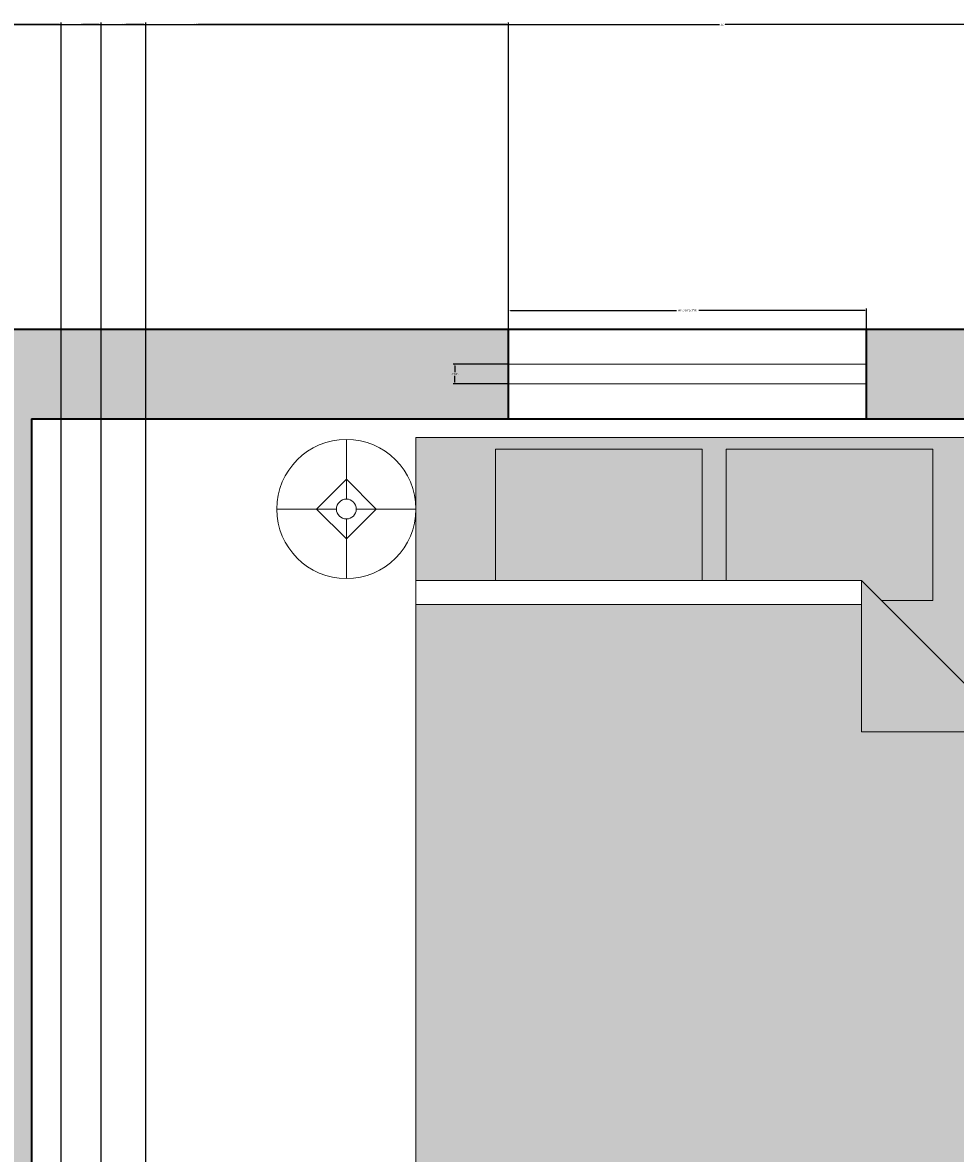
# Model space of a CAD drawing. Units: inches. Extents: x 1567 to 1964, y 1813 to 2447.
# Tile 27 of 28: x 1792 to 1885, y 2333 to 2447. Entities that reach past the tile are written whole.
import ezdxf

# ---------------------------------------------------------------- set-up
doc = ezdxf.new("R2010")
doc.units = ezdxf.units.IN
for name, color, linetype, lineweight in [('A-ANNO-DIMS', 2, 'Continuous', 18), ('A-FURN', 8, 'Continuous', 18), ('A-GLAZ', 4, 'Continuous', 18), ('A-WALL', 7, 'Continuous', 35)]:
    doc.layers.add(name, color=color, linetype=linetype, lineweight=lineweight)
doc.layers.add('A-FURN-PATT', color=252, linetype='Continuous', lineweight=13, true_color=0x939598)
doc.layers.add('A-WALL-PATT', color=251, linetype='Continuous', lineweight=13, true_color=0x636466)
doc.styles.get("Standard").update_dxf_attribs({"font": 'arial.ttf'})
doc.dimstyles.get("Standard").update_dxf_attribs({"dimtxt": 0.18, "dimasz": 0.18, "dimexe": 0.18, "dimexo": 0.0625, "dimgap": 0.09, "dimtad": 0, "dimtih": 1, "dimtoh": 1, "dimdec": 4, "dimzin": 0, "dimdsep": 46, "dimtxsty": 'Standard', "dimcen": 0.09, "dimadec": 0, "dimazin": 0, "dimtfac": 1, "dimtdec": 4, "dimtofl": 0, "dimtmove": 0, "dimatfit": 3, "dimfxl": 1, "dimtolj": 1, "dimtzin": 0, "dimarcsym": 0})

# ---------------------------------------------------------------- blocks, each defined once
blk = doc.blocks.new('Lamp - Table')
for p, q in [((0, 7), (0, 1)), ((0, 3), (-3, 0)), ((3, 0), (0, 3)), ((-1, 0), (-7, 0)), ((-3, 0), (0, -3)), ((0, -3), (3, 0)), ((1, 0), (7, 0)), ((0, -1), (0, -7))]:
    blk.add_line(p, q)
for radius in [7, 1]:
    blk.add_circle((0, 0), radius)
blk = doc.blocks.new('Bed - Queen')
for p, q in [((0, -80.00003), (0, 0)), ((0, 0), (59.99999, 0)), ((59.99999, 0), (59.99999, -80.00003)), ((7.99999, -1.2), (28.79998, -1.2)), ((7.99999, -14.4), (7.99999, -1.2)), ((28.79998, -1.2), (28.79998, -14.4)), ((31.19999, -1.2), (51.99999, -1.2)), ((31.19999, -14.4), (31.19999, -1.2)), ((51.99999, -1.2), (51.99999, -16.4)), ((0, -14.4), (44.8, -14.4)), ((59.99999, -29.6), (44.8, -14.4)), ((44.8, -14.4), (44.8, -29.6)), ((44.8, -16.8), (0, -16.8)), ((51.99999, -16.4), (46.79936, -16.4)), ((44.8, -29.6), (59.99999, -29.6)), ((59.99999, -80.00003), (0, -80.00003))]:
    blk.add_line(p, q)
blk = doc.blocks.new('WINDOW-36IN')
for p, q in [((0, 2), (36, 2)), ((0, 0), (36, 0))]:
    blk.add_line(p, q)
blk = doc.blocks.new('*D33')
at = {"layer": 'A-ANNO-DIMS', "color": 0, "lineweight": -2, "transparency": 16777216}
for p, q in [((1840.43, 2412.85), (1840.43, 2418.37)), ((1840.61, 2418.19), (1857.31, 2418.19)), ((1876.25, 2418.19), (1859.55, 2418.19)), ((1876.43, 2412.85), (1876.43, 2418.37))]:
    blk.add_line(p, q, dxfattribs=at)
at = {"layer": 'A-ANNO-DIMS', "color": 0, "transparency": 16777216}
for points in [[(1840.61, 2418.22), (1840.61, 2418.16), (1840.43, 2418.19)], [(1876.25, 2418.22), (1876.25, 2418.16), (1876.43, 2418.19)]]:
    blk.add_solid(points, dxfattribs=at)
at = {"layer": 'Defpoints', "color": 0, "transparency": 16777216}
for p in [(1840.43, 2418.19), (1840.43, 2412.79), (1876.43, 2412.79)]:
    blk.add_point(p, dxfattribs=at)
at = {"layer": 'A-ANNO-DIMS', "color": 0, "transparency": 16777216, "insert": (1858.43, 2418.19), "char_height": 0.18, "attachment_point": 5}
blk.add_mtext('\\A1;WINDOW 36 TYP.', dxfattribs=at)
blk = doc.blocks.new('*D34')
at = {"layer": 'A-ANNO-DIMS', "color": 0, "lineweight": -2, "transparency": 16777216}
for p, q in [((1840.37, 2412.79), (1834.85, 2412.79)), ((1835.03, 2412.61), (1835.03, 2411.97)), ((1835.03, 2410.97), (1835.03, 2411.61)), ((1840.37, 2410.79), (1834.85, 2410.79))]:
    blk.add_line(p, q, dxfattribs=at)
at = {"layer": 'A-ANNO-DIMS', "color": 0, "transparency": 16777216}
for points in [[(1835, 2412.61), (1835.06, 2412.61), (1835.03, 2412.79)], [(1835, 2410.97), (1835.06, 2410.97), (1835.03, 2410.79)]]:
    blk.add_solid(points, dxfattribs=at)
at = {"layer": 'Defpoints', "color": 0, "transparency": 16777216}
for p in [(1840.43, 2412.79), (1835.03, 2410.79), (1840.43, 2410.79)]:
    blk.add_point(p, dxfattribs=at)
at = {"layer": 'A-ANNO-DIMS', "color": 0, "transparency": 16777216, "insert": (1835.03, 2411.79), "char_height": 0.18, "attachment_point": 5}
blk.add_mtext('\\A1;2 TYP.', dxfattribs=at)
blk = doc.blocks.new('*D45')
at = {"layer": 'A-ANNO-DIMS', "color": 0, "lineweight": -2, "transparency": 16777216}
for p, q in [((1777.43, 2416.35), (1777.43, 2447.12)), ((1777.61, 2446.94), (1808.71, 2446.94)), ((1840.25, 2446.94), (1809.15, 2446.94)), ((1840.43, 2416.35), (1840.43, 2447.12))]:
    blk.add_line(p, q, dxfattribs=at)
at = {"layer": 'A-ANNO-DIMS', "color": 0, "transparency": 16777216}
for points in [[(1777.61, 2446.97), (1777.61, 2446.91), (1777.43, 2446.94)], [(1840.25, 2446.97), (1840.25, 2446.91), (1840.43, 2446.94)]]:
    blk.add_solid(points, dxfattribs=at)
at = {"layer": 'Defpoints', "color": 0, "transparency": 16777216}
for p in [(1840.43, 2446.94), (1777.43, 2416.29), (1840.43, 2416.29)]:
    blk.add_point(p, dxfattribs=at)
at = {"layer": 'A-ANNO-DIMS', "color": 0, "transparency": 16777216, "insert": (1808.93, 2446.94), "char_height": 0.18, "attachment_point": 5}
blk.add_mtext('\\A1;63', dxfattribs=at)
blk = doc.blocks.new('*D54')
at = {"layer": 'A-ANNO-DIMS', "color": 0, "lineweight": -2, "transparency": 16777216}
for p, q in [((1711.43, 1964.35), (1711.43, 2447.12)), ((1711.61, 2446.94), (1753.21, 2446.94)), ((1795.25, 2446.94), (1753.65, 2446.94)), ((1795.43, 1964.35), (1795.43, 2447.12))]:
    blk.add_line(p, q, dxfattribs=at)
at = {"layer": 'A-ANNO-DIMS', "color": 0, "transparency": 16777216}
for points in [[(1711.61, 2446.97), (1711.61, 2446.91), (1711.43, 2446.94)], [(1795.25, 2446.97), (1795.25, 2446.91), (1795.43, 2446.94)]]:
    blk.add_solid(points, dxfattribs=at)
at = {"layer": 'Defpoints', "color": 0, "transparency": 16777216}
for p in [(1795.43, 2446.94), (1711.43, 1964.29), (1795.43, 1964.29)]:
    blk.add_point(p, dxfattribs=at)
at = {"layer": 'A-ANNO-DIMS', "color": 0, "transparency": 16777216, "insert": (1753.43, 2446.94), "char_height": 0.18, "attachment_point": 5}
blk.add_mtext('\\A1;84', dxfattribs=at)
blk = doc.blocks.new('*D55')
at = {"layer": 'A-ANNO-DIMS', "color": 0, "lineweight": -2, "transparency": 16777216}
for p, q in [((1795.43, 1964.35), (1795.43, 2447.12)), ((1795.61, 2446.94), (1797.28, 2446.94)), ((1799.25, 2446.94), (1797.58, 2446.94)), ((1799.43, 1967.35), (1799.43, 2447.12))]:
    blk.add_line(p, q, dxfattribs=at)
at = {"layer": 'A-ANNO-DIMS', "color": 0, "transparency": 16777216}
for points in [[(1795.61, 2446.97), (1795.61, 2446.91), (1795.43, 2446.94)], [(1799.25, 2446.97), (1799.25, 2446.91), (1799.43, 2446.94)]]:
    blk.add_solid(points, dxfattribs=at)
at = {"layer": 'Defpoints', "color": 0, "transparency": 16777216}
for p in [(1799.43, 2446.94), (1799.43, 1967.29), (1795.43, 1964.29)]:
    blk.add_point(p, dxfattribs=at)
at = {"layer": 'A-ANNO-DIMS', "color": 0, "transparency": 16777216, "insert": (1797.43, 2446.94), "char_height": 0.18, "attachment_point": 5}
blk.add_mtext('\\A1;4', dxfattribs=at)
blk = doc.blocks.new('*D70')
at = {"layer": 'A-ANNO-DIMS', "color": 0, "lineweight": -2, "transparency": 16777216}
for p, q in [((1799.43, 1967.35), (1799.43, 2447.12)), ((1799.61, 2446.94), (1801.42, 2446.94)), ((1803.75, 2446.94), (1801.94, 2446.94)), ((1803.93, 1967.35), (1803.93, 2447.12))]:
    blk.add_line(p, q, dxfattribs=at)
at = {"layer": 'A-ANNO-DIMS', "color": 0, "transparency": 16777216}
for points in [[(1799.61, 2446.97), (1799.61, 2446.91), (1799.43, 2446.94)], [(1803.75, 2446.97), (1803.75, 2446.91), (1803.93, 2446.94)]]:
    blk.add_solid(points, dxfattribs=at)
at = {"layer": 'Defpoints', "color": 0, "transparency": 16777216}
for p in [(1803.93, 2446.94), (1799.43, 1967.29), (1803.93, 1967.29)]:
    blk.add_point(p, dxfattribs=at)
at = {"layer": 'A-ANNO-DIMS', "color": 0, "transparency": 16777216, "insert": (1801.68, 2446.94), "char_height": 0.18, "attachment_point": 5}
blk.add_mtext('\\A1;4.5', dxfattribs=at)
blk = doc.blocks.new('*D71')
at = {"layer": 'A-ANNO-DIMS', "color": 0, "lineweight": -2, "transparency": 16777216}
for p, q in [((1799.43, 1910.75), (1799.43, 2447.12)), ((1799.61, 2446.94), (1861.65, 2446.94)), ((1924.25, 2446.94), (1862.21, 2446.94)), ((1924.43, 1910.75), (1924.43, 2447.12))]:
    blk.add_line(p, q, dxfattribs=at)
at = {"layer": 'A-ANNO-DIMS', "color": 0, "transparency": 16777216}
for points in [[(1799.61, 2446.97), (1799.61, 2446.91), (1799.43, 2446.94)], [(1924.25, 2446.97), (1924.25, 2446.91), (1924.43, 2446.94)]]:
    blk.add_solid(points, dxfattribs=at)
at = {"layer": 'Defpoints', "color": 0, "transparency": 16777216}
for p in [(1924.43, 2446.94), (1799.43, 1910.69), (1924.43, 1910.69)]:
    blk.add_point(p, dxfattribs=at)
at = {"layer": 'A-ANNO-DIMS', "color": 0, "transparency": 16777216, "insert": (1861.93, 2446.94), "char_height": 0.18, "attachment_point": 5}
blk.add_mtext('\\A1;125', dxfattribs=at)

msp = doc.modelspace()

# ---------------------------------------------------------------- hatches: boundary and pattern name
at = {"layer": 'A-FURN-PATT'}
h = msp.add_hatch(color=256, dxfattribs=at)
h.dxf.hatch_style = 1
h.paths.add_polyline_path([(1621.2532, 2242.0229), (1643.7811, 2241.7239), (1643.8607, 2247.7234), (1617.863, 2248.0685, 0.19047621), (1616.7481, 2164.0759), (1642.7458, 2163.7308), (1642.8254, 2169.7302), (1620.2975, 2170.0293, -0.15194781)])
h.paths.add_polyline_path([(1673.5306, 2249.6607), (1653.8509, 2249.6607), (1653.8509, 2248.5031, 0.11764706), (1673.5306, 2248.5031)])
h.paths.add_polyline_path([(1706.0889, 2249.6607), (1686.4092, 2249.6607), (1686.4092, 2248.5031, 0.11764706), (1706.0889, 2248.5031)])
h.paths.add_polyline_path([(1782.4511, 2227.4197), (1766.4511, 2227.4197), (1766.2949, 2226.4197), (1782.6074, 2226.4197)])
h.paths.add_polyline_path([(1810.4511, 2227.4197), (1794.4511, 2227.4197), (1794.2949, 2226.4197), (1810.6074, 2226.4197)])
h.paths.add_polyline_path([(1743.9511, 2208.076), (1742.9511, 2207.9197), (1742.9511, 2191.9197), (1743.9511, 2191.7635)])
h.paths.add_polyline_path([(1782.6074, 2173.4197), (1766.2949, 2173.4197), (1766.4511, 2172.4197), (1782.4511, 2172.4197)])
h.paths.add_polyline_path([(1810.6074, 2173.4197), (1794.2949, 2173.4197), (1794.4511, 2172.4197), (1810.4511, 2172.4197)])
h.paths.add_polyline_path([(1861.053, 2006.5071), (1845.8531, 2006.5071), (1861.053, 1991.3071)])
h.paths.add_polyline_path([(1905.853, 1993.7071), (1861.053, 1993.7071), (1861.053, 1991.3071), (1905.853, 1991.3071)])
h.paths.add_polyline_path([(1919.7245, 2257.29, 0.50000012), (1918.7245, 2258.29), (1901.7245, 2258.29, 0.50000012), (1900.7245, 2257.29), (1900.7245, 2253.29, 0.50000012), (1901.7245, 2252.29), (1918.7245, 2252.29, 0.50000012), (1919.7245, 2253.29)])
h.paths.add_polyline_path([(1875.9094, 2391.0204), (1875.9094, 2375.8204), (1891.1093, 2375.8204)], flags=17)
h.paths.add_polyline_path([(1891.1093, 2405.4204), (1831.1094, 2405.4204), (1831.1094, 2391.0204), (1839.1093, 2391.0204), (1839.1093, 2404.2204), (1859.9093, 2404.2204), (1859.9093, 2391.0204), (1862.3093, 2391.0204), (1862.3093, 2404.2204), (1883.1093, 2404.2204), (1883.1093, 2389.0204), (1877.9094, 2389.0204), (1891.1093, 2375.8204)])
h.paths.add_polyline_path([(1682.1402, 2390.0316), (1682.1402, 2374.8316), (1697.3402, 2374.8316)], flags=17)
h.paths.add_polyline_path([(1697.3402, 2404.4316), (1637.3402, 2404.4316), (1637.3402, 2390.0316), (1645.3402, 2390.0316), (1645.3402, 2403.2316), (1666.1402, 2403.2316), (1666.1402, 2390.0316), (1668.5402, 2390.0316), (1668.5402, 2403.2316), (1689.3402, 2403.2316), (1689.3402, 2388.0316), (1684.1402, 2388.0316), (1697.3402, 2374.8316)])
h = msp.add_hatch(color=256, dxfattribs=at)
h.dxf.hatch_style = 1
h.paths.add_polyline_path([(1666.1402, 2403.2316), (1645.3402, 2403.2316), (1645.3402, 2390.0316), (1666.1402, 2390.0316)])
h.paths.add_polyline_path([(1689.3402, 2403.2316), (1668.5402, 2403.2316), (1668.5402, 2390.0316), (1682.1402, 2390.0316), (1684.1402, 2388.0316), (1689.3402, 2388.0316)])
h.paths.add_polyline_path([(1859.9093, 2404.2204), (1839.1093, 2404.2204), (1839.1093, 2391.0204), (1859.9093, 2391.0204)])
h.paths.add_polyline_path([(1883.1093, 2404.2204), (1862.3093, 2404.2204), (1862.3093, 2391.0204), (1875.9094, 2391.0204), (1877.9094, 2389.0204), (1883.1093, 2389.0204)])
h = msp.add_hatch(color=256, dxfattribs=at)
h.dxf.hatch_style = 1
h.paths.add_polyline_path([(1697.3402, 2374.8316), (1682.1402, 2374.8316), (1682.1402, 2387.6316), (1637.3402, 2387.6316), (1637.3402, 2324.4315), (1697.3402, 2324.4315)])
h.paths.add_polyline_path([(1891.1093, 2375.8204), (1875.9094, 2375.8204), (1875.9094, 2388.6204), (1831.1094, 2388.6204), (1831.1094, 2325.4204), (1891.1093, 2325.4204)])
h.paths.add_polyline_path([(1702.5611, 2206.8057), (1702.5611, 2210.8057), (1699.7395, 2209.9436), (1697.013, 2209.2403), (1694.3857, 2208.6763), (1691.8615, 2208.2326), (1689.4443, 2207.8896), (1687.1381, 2207.6282), (1684.9469, 2207.4289), (1682.8747, 2207.2725), (1680.9233, 2207.1425), (1679.0865, 2207.0339), (1677.3558, 2206.9445), (1675.7229, 2206.8719), (1674.1794, 2206.8141), (1672.7169, 2206.7688), (1671.327, 2206.7339), (1670.0014, 2206.707), (1668.7314, 2206.6866), (1667.5072, 2206.6732), (1666.3188, 2206.668), (1665.1561, 2206.6722), (1664.009, 2206.6869), (1662.8675, 2206.7133), (1661.7215, 2206.7525), (1660.5611, 2206.8057), (1660.5611, 2202.8057), (1661.9932, 2202.9556), (1663.3314, 2203.0744), (1664.5899, 2203.1671), (1665.7831, 2203.2385), (1666.9254, 2203.2935), (1668.0311, 2203.3368), (1669.1145, 2203.3734), (1670.1902, 2203.4081), (1671.2724, 2203.4451), (1672.3759, 2203.4866), (1673.5155, 2203.534), (1674.706, 2203.5887), (1675.9621, 2203.6523), (1677.2986, 2203.7262), (1678.7304, 2203.8118), (1680.2722, 2203.9108), (1681.947, 2204.0272), (1683.8108, 2204.1769), (1685.9279, 2204.3782), (1688.3626, 2204.6496), (1691.179, 2205.0096), (1694.4413, 2205.4767), (1698.214, 2206.0692)])
h.paths.add_polyline_path([(1702.5611, 2218.8057), (1701.9821, 2217.9383), (1701.3316, 2217.191), (1700.6091, 2216.5515), (1699.8141, 2216.0071), (1698.946, 2215.5454), (1698.0041, 2215.1536), (1696.9879, 2214.8194), (1695.8969, 2214.5301), (1694.7328, 2214.2753), (1693.5072, 2214.0522), (1692.2339, 2213.8602), (1690.9266, 2213.6989), (1689.5994, 2213.5675), (1688.266, 2213.4654), (1686.9402, 2213.392), (1685.636, 2213.3467), (1684.3619, 2213.3287), (1683.1053, 2213.3361), (1681.8482, 2213.3668), (1680.5727, 2213.4187), (1679.2608, 2213.4898), (1677.8948, 2213.5779), (1676.4565, 2213.6811), (1674.9282, 2213.7971), (1673.2982, 2213.9236), (1671.5804, 2214.0573), (1669.795, 2214.1945), (1667.9622, 2214.3316), (1666.1022, 2214.4649), (1664.2352, 2214.5908), (1662.3814, 2214.7056), (1660.5611, 2214.8057), (1660.5611, 2206.8057), (1661.7215, 2206.7525), (1662.8675, 2206.7133), (1664.009, 2206.6869), (1665.1561, 2206.6722), (1666.3188, 2206.668), (1667.5072, 2206.6732), (1668.7314, 2206.6866), (1670.0014, 2206.707), (1671.327, 2206.7339), (1672.7169, 2206.7688), (1674.1794, 2206.8141), (1675.7229, 2206.8719), (1677.3558, 2206.9445), (1679.0865, 2207.0339), (1680.9233, 2207.1425), (1682.8747, 2207.2725), (1684.9469, 2207.4289), (1687.1381, 2207.6282), (1689.4443, 2207.8896), (1691.8615, 2208.2326), (1694.3857, 2208.6763), (1697.013, 2209.2403), (1699.7395, 2209.9436), (1702.5611, 2210.8057)])
h.paths.add_polyline_path([(1700.6091, 2216.5515), (1701.3316, 2217.191), (1701.9821, 2217.9383), (1702.5611, 2218.8057), (1702.5611, 2222.8057), (1689.452, 2222.8057), (1689.0171, 2222.4556), (1688.4521, 2222.0354), (1687.7806, 2221.5662), (1687.0235, 2221.067), (1686.2019, 2220.5566), (1685.3367, 2220.0541), (1684.4491, 2219.5785), (1683.56, 2219.1486), (1682.6867, 2218.7795), (1681.8312, 2218.4692), (1680.9918, 2218.212), (1680.1667, 2218.0019), (1679.3541, 2217.833), (1678.5524, 2217.6995), (1677.7597, 2217.5954), (1676.9744, 2217.5149), (1676.1942, 2217.4531), (1675.4146, 2217.4093), (1674.6309, 2217.384), (1673.8381, 2217.3774), (1673.0313, 2217.39), (1672.2056, 2217.4221), (1671.3562, 2217.4741), (1670.4782, 2217.5463), (1669.5642, 2217.639), (1668.5968, 2217.7516), (1667.5562, 2217.8833), (1666.4226, 2218.0336), (1665.1761, 2218.2017), (1663.7969, 2218.3869), (1662.2651, 2218.5885), (1660.5611, 2218.8057), (1660.5611, 2214.8057), (1662.3814, 2214.7056), (1664.2352, 2214.5908), (1666.1022, 2214.4649), (1667.9622, 2214.3316), (1669.795, 2214.1945), (1671.5804, 2214.0573), (1673.2982, 2213.9236), (1674.9282, 2213.7971), (1676.4565, 2213.6811), (1677.8948, 2213.5779), (1679.2608, 2213.4898), (1680.5727, 2213.4187), (1681.8482, 2213.3668), (1683.1053, 2213.3361), (1684.3619, 2213.3287), (1685.636, 2213.3467), (1686.9402, 2213.392), (1688.266, 2213.4654), (1689.5994, 2213.5675), (1690.9266, 2213.6989), (1692.2339, 2213.8602), (1693.5072, 2214.0522), (1694.7328, 2214.2753), (1695.8969, 2214.5301), (1696.9879, 2214.8194), (1698.0041, 2215.1536), (1698.946, 2215.5454), (1699.8141, 2216.0071)])
h.paths.add_polyline_path([(1687.0235, 2221.067), (1687.7806, 2221.5662), (1688.4521, 2222.0354), (1689.0171, 2222.4556), (1689.452, 2222.8057), (1660.5611, 2222.8057), (1660.5611, 2218.8057), (1662.2651, 2218.5885), (1663.7969, 2218.3869), (1665.1761, 2218.2017), (1666.4226, 2218.0336), (1667.5562, 2217.8833), (1668.5968, 2217.7516), (1669.5642, 2217.639), (1670.4782, 2217.5463), (1671.3562, 2217.4741), (1672.2056, 2217.4221), (1673.0313, 2217.39), (1673.8381, 2217.3774), (1674.6309, 2217.384), (1675.4146, 2217.4093), (1676.1942, 2217.4531), (1676.9744, 2217.5149), (1677.7597, 2217.5954), (1678.5524, 2217.6995), (1679.3541, 2217.833), (1680.1667, 2218.0019), (1680.9918, 2218.212), (1681.8312, 2218.4692), (1682.6867, 2218.7795), (1683.56, 2219.1486), (1684.4491, 2219.5785), (1685.3367, 2220.0541), (1686.2019, 2220.5566)], flags=17)
h.paths.add_polyline_path([(1702.5611, 2198.8057), (1698.9289, 2199.2412), (1695.8472, 2199.5774), (1693.2166, 2199.8257), (1690.9377, 2199.9973), (1688.9111, 2200.1033), (1687.0375, 2200.155), (1685.2174, 2200.1637), (1683.3514, 2200.1406), (1681.3514, 2200.0941), (1679.1736, 2200.0225), (1676.7858, 2199.921), (1674.1554, 2199.7852), (1671.2502, 2199.6103), (1668.0377, 2199.3919), (1664.4854, 2199.1252), (1660.5611, 2198.8057), (1660.5611, 2194.8057), (1662.2697, 2194.9771), (1663.9673, 2195.0999), (1665.6339, 2195.1809), (1667.2495, 2195.227), (1668.7941, 2195.2449), (1670.2478, 2195.2414), (1671.5906, 2195.2233), (1672.8026, 2195.1974), (1673.8739, 2195.1689), (1674.8359, 2195.1364), (1675.7302, 2195.0967), (1676.5982, 2195.0469), (1677.4817, 2194.9838), (1678.422, 2194.9043), (1679.4609, 2194.8055), (1680.6397, 2194.6842), (1682.005, 2194.5341), (1683.6223, 2194.335), (1685.562, 2194.0637), (1687.8945, 2193.6967), (1690.6902, 2193.2108), (1694.0196, 2192.5826), (1697.9531, 2191.7887), (1702.5611, 2190.8057)])
h.paths.add_polyline_path([(1702.5611, 2206.8057), (1698.214, 2206.0692), (1694.4413, 2205.4767), (1691.179, 2205.0096), (1688.3626, 2204.6496), (1685.9279, 2204.3782), (1683.8108, 2204.1769), (1681.947, 2204.0272), (1680.2722, 2203.9108), (1678.7304, 2203.8118), (1677.2986, 2203.7262), (1675.9621, 2203.6523), (1674.706, 2203.5887), (1673.5155, 2203.534), (1672.3759, 2203.4866), (1671.2724, 2203.4451), (1670.1902, 2203.4081), (1669.1145, 2203.3734), (1668.0311, 2203.3368), (1666.9254, 2203.2935), (1665.7831, 2203.2385), (1664.5899, 2203.1671), (1663.3314, 2203.0744), (1661.9932, 2202.9556), (1660.5611, 2202.8057), (1660.5611, 2198.8057), (1664.4854, 2199.1252), (1668.0377, 2199.3919), (1671.2502, 2199.6103), (1674.1554, 2199.7852), (1676.7858, 2199.921), (1679.1736, 2200.0225), (1681.3514, 2200.0941), (1683.3514, 2200.1406), (1685.2174, 2200.1637), (1687.0375, 2200.155), (1688.9111, 2200.1033), (1690.9377, 2199.9973), (1693.2166, 2199.8257), (1695.8472, 2199.5774), (1698.9289, 2199.2412), (1702.5611, 2198.8057)])
h.paths.add_polyline_path([(1702.5611, 2190.8057), (1697.9531, 2191.7887), (1694.0196, 2192.5826), (1690.6902, 2193.2108), (1687.8945, 2193.6967), (1685.562, 2194.0637), (1683.6223, 2194.335), (1682.005, 2194.5341), (1680.6397, 2194.6842), (1679.4609, 2194.8055), (1678.422, 2194.9043), (1677.4817, 2194.9838), (1676.5982, 2195.0469), (1675.7302, 2195.0967), (1674.8359, 2195.1364), (1673.8739, 2195.1689), (1672.8026, 2195.1974), (1671.5906, 2195.2233), (1670.2478, 2195.2414), (1668.7941, 2195.2449), (1667.2495, 2195.227), (1665.6339, 2195.1809), (1663.9673, 2195.0999), (1662.2697, 2194.9771), (1660.5611, 2194.8057), (1660.5611, 2190.8057), (1665.9637, 2190.2699), (1670.5105, 2189.7867), (1674.3035, 2189.3504), (1677.4445, 2188.9552), (1680.0354, 2188.5951), (1682.1782, 2188.2644), (1683.9747, 2187.9571), (1685.5268, 2187.6675), (1686.9225, 2187.3901), (1688.1943, 2187.1216), (1689.3606, 2186.859), (1690.4399, 2186.5993), (1691.4508, 2186.3396), (1692.4118, 2186.0769), (1693.3413, 2185.8084), (1694.2579, 2185.531), (1695.1786, 2185.2422), (1696.1142, 2184.9406), (1697.0739, 2184.6252), (1698.0671, 2184.2949), (1699.1032, 2183.9489), (1700.1913, 2183.586), (1701.3408, 2183.2053), (1702.5611, 2182.8057)])
h.paths.add_polyline_path([(1702.5611, 2182.8057), (1701.3408, 2183.2053), (1700.1913, 2183.586), (1699.1032, 2183.9489), (1698.0671, 2184.2949), (1697.0739, 2184.6252), (1696.1142, 2184.9406), (1695.1786, 2185.2422), (1694.2579, 2185.531), (1693.3413, 2185.8084), (1692.4118, 2186.0769), (1691.4508, 2186.3396), (1690.4399, 2186.5993), (1689.3606, 2186.859), (1688.1943, 2187.1216), (1686.9225, 2187.3901), (1685.5268, 2187.6675), (1683.9747, 2187.9571), (1682.1782, 2188.2644), (1680.0354, 2188.5951), (1677.4445, 2188.9552), (1674.3035, 2189.3504), (1670.5105, 2189.7867), (1665.9637, 2190.2699), (1660.5611, 2190.8057), (1660.5611, 2186.8057), (1663.5709, 2186.52), (1666.0965, 2186.2414), (1668.1979, 2185.9698), (1669.9351, 2185.7048), (1671.3681, 2185.446), (1672.5568, 2185.1931), (1673.5613, 2184.9458), (1674.4415, 2184.7037), (1675.2485, 2184.4664), (1675.9976, 2184.2328), (1677.0295, 2183.8907), (1678.2492, 2183.4332), (1679.354, 2182.9669), (1680.4123, 2182.4724), (1681.3757, 2181.9718), (1682.2435, 2181.4594), (1683.1864, 2180.8057), (1702.5611, 2180.8057)])
h.paths.add_polyline_path([(1677.3469, 2183.7716), (1676.6949, 2184.0016), (1675.9976, 2184.2328), (1675.2485, 2184.4664), (1674.4415, 2184.7037), (1673.5613, 2184.9458), (1672.5568, 2185.1931), (1671.3681, 2185.446), (1669.9351, 2185.7048), (1668.1979, 2185.9698), (1666.0965, 2186.2414), (1663.5709, 2186.52), (1660.5611, 2186.8057), (1660.5611, 2180.8057), (1683.1506, 2180.8057), (1682.802, 2181.0722), (1682.4264, 2181.3326), (1682.0201, 2181.5913), (1681.586, 2181.8476), (1681.1268, 2182.1011), (1680.6453, 2182.3513), (1680.1443, 2182.5976), (1679.6266, 2182.8395), (1679.0933, 2183.0769), (1678.5398, 2183.3105), (1677.9598, 2183.5417)], flags=17)
h.paths.add_polyline_path([(1824.4511, 2199.9016), (1824.089, 2199.9302), (1824.0595, 2199.9372), (1824.0397, 2199.9406), (1823.5413, 2200.0576), (1823.4095, 2200.0864), (1823.0664, 2200.1559), (1822.6419, 2200.2361), (1822.1519, 2200.3222), (1821.6126, 2200.4093), (1821.0401, 2200.4925), (1820.4505, 2200.5669), (1819.8599, 2200.6276), (1819.2845, 2200.6697), (1818.7366, 2200.6896), (1818.2141, 2200.688), (1817.7112, 2200.6668), (1817.222, 2200.6281), (1816.7405, 2200.5737), (1816.261, 2200.5057), (1815.7776, 2200.4259), (1815.2845, 2200.3364), (1814.3007, 2200.149), (1813.3315, 2199.9765), (1812.406, 2199.8514), (1811.6868, 2199.7739), (1810.8992, 2199.7121), (1810.0345, 2199.6697), (1809.0854, 2199.6497), (1808.0514, 2199.6502), (1806.9334, 2199.6683), (1805.7324, 2199.701), (1804.4493, 2199.7454), (1803.0852, 2199.7986), (1801.641, 2199.8577), (1800.1178, 2199.9197), (1798.5134, 2199.9818), (1796.8144, 2200.0415), (1795.004, 2200.0962), (1793.0657, 2200.1437), (1790.9828, 2200.1814), (1788.7389, 2200.2068), (1786.3171, 2200.2177), (1783.7011, 2200.2114), (1780.8715, 2200.185), (1777.7988, 2200.1326), (1774.4506, 2200.0481), (1770.7948, 2199.9249), (1766.7992, 2199.7569), (1762.4316, 2199.5376), (1757.6596, 2199.2606), (1752.4511, 2198.9197), (1752.4511, 2193.4197), (1761.2668, 2193.6071), (1768.3671, 2193.7934), (1773.9821, 2193.9778), (1778.3417, 2194.1593), (1781.6759, 2194.3369), (1784.2148, 2194.5096), (1786.1882, 2194.6764), (1787.8261, 2194.8364), (1789.3219, 2194.9887), (1790.7226, 2195.1333), (1792.0383, 2195.27), (1793.2792, 2195.3989), (1794.4557, 2195.52), (1795.5781, 2195.6333), (1796.6564, 2195.7387), (1797.7011, 2195.8364), (1798.7216, 2195.9259), (1799.7245, 2196.0057), (1800.7158, 2196.0737), (1801.7011, 2196.1281), (1802.6865, 2196.1668), (1803.6777, 2196.188), (1804.6806, 2196.1896), (1805.7011, 2196.1697), (1806.7423, 2196.1273), (1807.7962, 2196.0643), (1808.852, 2195.9837), (1809.899, 2195.8885), (1810.9265, 2195.7815), (1811.9238, 2195.6658), (1812.88, 2195.5442), (1813.7845, 2195.4197), (1814.6296, 2195.2948), (1815.4205, 2195.1704), (1816.1656, 2195.0469), (1816.873, 2194.9249), (1817.5511, 2194.8049), (1818.2083, 2194.6873), (1818.8527, 2194.5726), (1819.4928, 2194.4614), (1820.1348, 2194.3554), (1820.7773, 2194.2615), (1821.4169, 2194.1882), (1822.0501, 2194.1437), (1822.6735, 2194.1363), (1823.2838, 2194.1743), (1823.8775, 2194.266), (1824.4511, 2194.4197)])
h.paths.add_polyline_path([(1821.4716, 2190.5098), (1820.4303, 2190.5708), (1819.3811, 2190.6415), (1818.3339, 2190.7186), (1817.2985, 2190.7986), (1816.2845, 2190.8781), (1815.2976, 2190.9542), (1814.3274, 2191.0259), (1813.3592, 2191.0927), (1812.3782, 2191.1541), (1811.3699, 2191.2097), (1810.3196, 2191.2589), (1809.2127, 2191.3013), (1808.0345, 2191.3364), (1806.7708, 2191.3634), (1805.4094, 2191.3807), (1803.9387, 2191.3862), (1802.3469, 2191.3781), (1800.6223, 2191.3543), (1798.7532, 2191.313), (1796.7278, 2191.2521), (1794.5344, 2191.1697), (1792.128, 2191.0648), (1789.33, 2190.9393), (1785.9285, 2190.7962), (1781.7115, 2190.6385), (1776.4672, 2190.469), (1769.9836, 2190.2908), (1762.0489, 2190.1067), (1752.4511, 2189.9197), (1752.4511, 2185.4197), (1758.363, 2185.5846), (1763.4179, 2185.7075), (1767.7199, 2185.7933), (1771.373, 2185.8468), (1774.4811, 2185.873), (1777.1484, 2185.8768), (1779.4787, 2185.8629), (1781.5761, 2185.8364), (1783.5287, 2185.8014), (1785.3606, 2185.7596), (1787.0802, 2185.7119), (1788.6959, 2185.6593), (1790.2158, 2185.6028), (1791.6484, 2185.5434), (1793.0018, 2185.4821), (1794.2844, 2185.4197), (1795.5065, 2185.3576), (1796.6861, 2185.298), (1797.8433, 2185.2432), (1798.998, 2185.1958), (1800.1703, 2185.1581), (1801.3801, 2185.1326), (1802.6476, 2185.1218), (1803.9928, 2185.1281), (1805.4444, 2185.1555), (1807.0663, 2185.2147), (1808.9315, 2185.3178), (1811.1126, 2185.477), (1813.6823, 2185.7046), (1816.7135, 2186.0128), (1820.2788, 2186.4138), (1824.4511, 2186.9197), (1824.4511, 2190.4197), (1823.4918, 2190.4309), (1822.4954, 2190.4621)])
h.paths.add_polyline_path([(1797.3762, 2216.0584), (1797.6199, 2216.2267), (1797.9558, 2216.3355), (1798.3017, 2216.3703), (1798.5761, 2216.3781), (1798.8974, 2216.3703), (1799.2714, 2216.3468), (1799.704, 2216.3078), (1800.2011, 2216.2531), (1800.7695, 2216.1829), (1801.4205, 2216.0981), (1802.1662, 2215.9996), (1803.0188, 2215.8885), (1803.9906, 2215.7656), (1805.0937, 2215.632), (1806.3404, 2215.4886), (1807.7428, 2215.3364), (1809.3101, 2215.1764), (1811.039, 2215.0096), (1812.9232, 2214.8369), (1814.9563, 2214.6593), (1817.132, 2214.4778), (1819.444, 2214.2934), (1821.8858, 2214.1071), (1824.4511, 2213.9197), (1824.4511, 2217.9197), (1752.4511, 2217.9197), (1752.4511, 2214.9197), (1757.2739, 2214.8973), (1761.6432, 2214.8338), (1765.5973, 2214.7352), (1769.1751, 2214.6072), (1772.4149, 2214.4559), (1775.3554, 2214.2869), (1778.0352, 2214.1063), (1780.4928, 2213.9197), (1782.7607, 2213.7329), (1784.8476, 2213.5499), (1786.7557, 2213.3748), (1788.4876, 2213.2114), (1790.0456, 2213.0636), (1791.4322, 2212.9354), (1792.6499, 2212.8305), (1793.7011, 2212.7531), (1794.5904, 2212.7059), (1795.3313, 2212.688), (1795.9394, 2212.6974), (1796.4303, 2212.7322), (1796.8196, 2212.7905), (1797.123, 2212.8703), (1797.356, 2212.9695), (1797.5344, 2213.0864), (1797.6716, 2213.2187), (1797.7727, 2213.3637), (1797.8406, 2213.5185), (1797.8782, 2213.6801), (1797.8884, 2213.8457), (1797.8743, 2214.0122), (1797.8386, 2214.1767), (1797.7844, 2214.3364), (1797.7149, 2214.4889), (1797.6347, 2214.6346), (1797.5486, 2214.7744), (1797.3327, 2215.109), (1797.178, 2215.4303), (1797.1896, 2215.7939)])
h.paths.add_polyline_path([(1804.7872, 2210.6789), (1804.546, 2211.022), (1804.3512, 2211.3917), (1804.2466, 2211.7546), (1804.2574, 2212.0998), (1804.4058, 2212.4178), (1804.7068, 2212.7007), (1805.1359, 2212.9124), (1805.5279, 2212.9926), (1805.8136, 2213.0154), (1806.1178, 2213.0031), (1806.4405, 2212.9529), (1806.7929, 2212.867), (1807.1893, 2212.7489), (1807.6438, 2212.602), (1808.1706, 2212.4297), (1808.7838, 2212.2355), (1809.4976, 2212.0227), (1810.3261, 2211.7947), (1811.2868, 2211.5533), (1812.4101, 2211.2928), (1813.7297, 2211.0059), (1815.2793, 2210.6854), (1817.0925, 2210.3238), (1819.2031, 2209.9139), (1821.6447, 2209.4483), (1824.4511, 2208.9197), (1824.4511, 2213.9197), (1821.8858, 2214.1071), (1819.444, 2214.2934), (1817.132, 2214.4778), (1814.9563, 2214.6593), (1812.9232, 2214.8369), (1811.039, 2215.0096), (1809.3101, 2215.1764), (1807.7428, 2215.3364), (1806.3404, 2215.4886), (1805.0937, 2215.632), (1803.9906, 2215.7656), (1803.0188, 2215.8885), (1802.1662, 2215.9996), (1801.4205, 2216.0981), (1800.7695, 2216.1829), (1800.2011, 2216.2531), (1799.704, 2216.3078), (1799.2714, 2216.3468), (1798.8974, 2216.3703), (1798.5761, 2216.3781), (1798.3017, 2216.3703), (1798.0683, 2216.3468), (1797.87, 2216.3078), (1797.7011, 2216.2531), (1797.5566, 2216.1831), (1797.4355, 2216.0994), (1797.3378, 2216.004), (1797.2636, 2215.8989), (1797.2128, 2215.7859), (1797.1855, 2215.6671), (1797.1816, 2215.5444), (1797.2011, 2215.4197), (1797.2433, 2215.2946), (1797.304, 2215.1684), (1797.3783, 2215.0403), (1797.4615, 2214.9093), (1797.6718, 2214.5836), (1797.8218, 2214.2545), (1797.8933, 2213.9247), (1797.8728, 2213.5918), (1797.7366, 2213.2814), (1797.4586, 2213.0132), (1797.123, 2212.8703), (1796.8196, 2212.7905), (1796.4303, 2212.7322), (1795.9394, 2212.6974), (1795.3313, 2212.688), (1794.5904, 2212.7059), (1793.7011, 2212.7531), (1792.6499, 2212.8305), (1791.4322, 2212.9354), (1790.0456, 2213.0636), (1788.4876, 2213.2114), (1786.7557, 2213.3748), (1784.8476, 2213.5499), (1782.7607, 2213.7329), (1780.4928, 2213.9197), (1778.0352, 2214.1063), (1775.3554, 2214.2869), (1772.4149, 2214.4559), (1769.1751, 2214.6072), (1765.5973, 2214.7352), (1761.6432, 2214.8338), (1757.2739, 2214.8973), (1752.4511, 2214.9197), (1752.4511, 2209.9197), (1759.4745, 2210.0625), (1765.2786, 2210.1242), (1770.027, 2210.1175), (1773.8834, 2210.0551), (1777.0112, 2209.9498), (1779.5741, 2209.8143), (1781.7357, 2209.6611), (1783.6594, 2209.5031), (1785.4813, 2209.3506), (1787.2265, 2209.2049), (1788.8926, 2209.0651), (1790.4771, 2208.9301), (1791.9777, 2208.7991), (1793.3919, 2208.671), (1794.7171, 2208.5449), (1795.9511, 2208.4197), (1797.0922, 2208.2952), (1798.1425, 2208.1736), (1799.1049, 2208.0579), (1799.9823, 2207.951), (1800.7778, 2207.8558), (1801.4941, 2207.7752), (1802.1342, 2207.7122), (1802.7011, 2207.6697), (1803.1982, 2207.65), (1803.6308, 2207.6528), (1804.0048, 2207.6771), (1804.3261, 2207.7218), (1804.6005, 2207.7861), (1804.8339, 2207.869), (1805.0322, 2207.9694), (1805.2011, 2208.0864), (1805.3455, 2208.2189), (1805.4654, 2208.365), (1805.56, 2208.5229), (1805.6282, 2208.6906), (1805.6691, 2208.866), (1805.6816, 2209.0473), (1805.6648, 2209.2326), (1805.6178, 2209.4197), (1805.5406, 2209.6072), (1805.4381, 2209.7947), (1805.316, 2209.9822), (1805.1803, 2210.1697), (1805.0367, 2210.3572)])
h.paths.add_polyline_path([(1801.4941, 2207.7752), (1800.7778, 2207.8558), (1799.9823, 2207.951), (1799.1049, 2208.0579), (1798.1425, 2208.1736), (1797.0922, 2208.2952), (1795.9511, 2208.4197), (1794.7171, 2208.5449), (1793.3919, 2208.671), (1791.9777, 2208.7991), (1790.4771, 2208.9301), (1788.8926, 2209.0651), (1787.2265, 2209.2049), (1785.4813, 2209.3506), (1783.6594, 2209.5031), (1781.7357, 2209.6611), (1779.5741, 2209.8143), (1777.0112, 2209.9498), (1773.8834, 2210.0551), (1770.027, 2210.1175), (1765.2786, 2210.1242), (1759.4745, 2210.0625), (1752.4511, 2209.9197), (1752.4511, 2205.4197), (1757.7354, 2205.2545), (1762.3821, 2205.1294), (1766.4565, 2205.0374), (1770.024, 2204.9718), (1773.1502, 2204.9258), (1775.9003, 2204.8924), (1778.3399, 2204.8649), (1780.5344, 2204.8364), (1782.5421, 2204.8014), (1784.3925, 2204.7596), (1786.1082, 2204.7119), (1787.7115, 2204.6593), (1789.225, 2204.6028), (1790.6711, 2204.5434), (1792.0724, 2204.4821), (1793.4511, 2204.4197), (1794.8241, 2204.3576), (1796.1855, 2204.2973), (1797.5234, 2204.241), (1798.8261, 2204.1906), (1800.082, 2204.1479), (1801.2792, 2204.115), (1802.4062, 2204.0939), (1803.4511, 2204.0864), (1804.4051, 2204.0942), (1805.2701, 2204.1176), (1806.0512, 2204.1567), (1806.7532, 2204.2114), (1807.381, 2204.2817), (1807.9394, 2204.3676), (1808.4334, 2204.4692), (1808.8678, 2204.5864), (1809.248, 2204.7187), (1809.5813, 2204.8637), (1809.8756, 2205.0185), (1810.1386, 2205.1801), (1810.3782, 2205.3457), (1810.6022, 2205.5122), (1810.9725, 2205.7941), (1811.3803, 2206.072), (1811.739, 2206.2612), (1812.0032, 2206.3781), (1812.2869, 2206.4793), (1812.5931, 2206.563), (1812.9246, 2206.6271), (1813.2845, 2206.6697), (1813.6746, 2206.6894), (1814.0931, 2206.6867), (1814.5369, 2206.6624), (1815.0032, 2206.6176), (1815.489, 2206.5534), (1815.9915, 2206.4705), (1816.5076, 2206.3701), (1817.0345, 2206.2531), (1817.5753, 2206.1196), (1818.1582, 2205.9666), (1818.8172, 2205.7902), (1819.5865, 2205.5864), (1820.5004, 2205.3514), (1821.5931, 2205.0812), (1822.8986, 2204.7719), (1824.4511, 2204.4197), (1824.4511, 2208.9197), (1821.6447, 2209.4483), (1819.2031, 2209.9139), (1817.0925, 2210.3238), (1815.2793, 2210.6854), (1813.7297, 2211.0059), (1812.4101, 2211.2928), (1811.2868, 2211.5533), (1810.3261, 2211.7947), (1809.4976, 2212.0227), (1808.7838, 2212.2355), (1808.1706, 2212.4297), (1807.6438, 2212.602), (1807.1893, 2212.7489), (1806.7929, 2212.867), (1806.4405, 2212.9529), (1806.1178, 2213.0031), (1805.8136, 2213.0154), (1805.5279, 2212.9926), (1805.2638, 2212.9386), (1805.024, 2212.8572), (1804.8116, 2212.7524), (1804.6295, 2212.6281), (1804.4806, 2212.4881), (1804.3678, 2212.3364), (1804.2931, 2212.1764), (1804.2545, 2212.0096), (1804.2491, 2211.8369), (1804.274, 2211.6593), (1804.3263, 2211.4778), (1804.4029, 2211.2934), (1804.5011, 2211.1071), (1804.6178, 2210.9197), (1804.7496, 2210.7322), (1804.8912, 2210.5447), (1805.154, 2210.2061), (1805.3962, 2209.8715), (1805.5964, 2209.5053), (1805.688, 2209.1402), (1805.6629, 2208.7758), (1805.5257, 2208.4385), (1805.2839, 2208.1437), (1804.9434, 2207.9078), (1804.6005, 2207.7861), (1804.3261, 2207.7218), (1804.0048, 2207.6771), (1803.6308, 2207.6528), (1803.1982, 2207.65), (1802.7011, 2207.6697), (1802.1342, 2207.7122)])
h.paths.add_polyline_path([(1824.4511, 2204.4197), (1822.8986, 2204.7719), (1821.5931, 2205.0812), (1820.5004, 2205.3514), (1819.5865, 2205.5864), (1818.8172, 2205.7902), (1818.1582, 2205.9666), (1817.5753, 2206.1196), (1817.0345, 2206.2531), (1816.5076, 2206.3701), (1815.9915, 2206.4705), (1815.489, 2206.5534), (1815.0032, 2206.6176), (1814.5369, 2206.6624), (1814.0931, 2206.6867), (1813.6746, 2206.6894), (1813.2845, 2206.6697), (1812.9246, 2206.6271), (1812.5931, 2206.563), (1812.2869, 2206.4793), (1812.0032, 2206.3781), (1811.739, 2206.2612), (1811.4915, 2206.1307), (1811.2576, 2205.9884), (1811.0345, 2205.8364), (1810.8183, 2205.6767), (1810.4357, 2205.3854), (1810.1386, 2205.1801), (1809.8756, 2205.0185), (1809.5813, 2204.8637), (1809.248, 2204.7187), (1808.8678, 2204.5864), (1808.4334, 2204.4692), (1807.9394, 2204.3676), (1807.381, 2204.2817), (1806.7532, 2204.2114), (1806.0512, 2204.1567), (1805.2701, 2204.1176), (1804.4051, 2204.0942), (1803.4511, 2204.0864), (1802.4062, 2204.0939), (1801.2792, 2204.115), (1800.082, 2204.1479), (1798.8261, 2204.1906), (1797.5234, 2204.241), (1796.1855, 2204.2973), (1794.8241, 2204.3576), (1793.4511, 2204.4197), (1792.0724, 2204.4821), (1790.6711, 2204.5434), (1789.225, 2204.6028), (1787.7115, 2204.6593), (1786.1082, 2204.7119), (1784.3925, 2204.7596), (1782.5421, 2204.8014), (1780.5344, 2204.8364), (1778.3399, 2204.8649), (1775.9003, 2204.8924), (1773.1502, 2204.9258), (1770.024, 2204.9718), (1766.4565, 2205.0374), (1762.3821, 2205.1294), (1757.7354, 2205.2545), (1752.4511, 2205.4197), (1752.4511, 2198.9197), (1757.6596, 2199.2606), (1762.4316, 2199.5376), (1766.7992, 2199.7569), (1770.7948, 2199.9249), (1774.4506, 2200.0481), (1777.7988, 2200.1326), (1780.8715, 2200.185), (1783.7011, 2200.2114), (1786.3171, 2200.2177), (1788.7389, 2200.2068), (1790.9828, 2200.1814), (1793.0657, 2200.1437), (1795.004, 2200.0962), (1796.8144, 2200.0415), (1798.5134, 2199.9818), (1800.1178, 2199.9197), (1801.641, 2199.8577), (1803.0852, 2199.7986), (1804.4493, 2199.7454), (1805.7324, 2199.701), (1806.9334, 2199.6683), (1808.0514, 2199.6502), (1809.0854, 2199.6497), (1810.0345, 2199.6697), (1810.8992, 2199.7121), (1811.6868, 2199.7739), (1812.406, 2199.8514), (1813.0657, 2199.9406), (1813.6746, 2200.0376), (1814.2415, 2200.1385), (1814.7752, 2200.2394), (1815.2845, 2200.3364), (1815.7776, 2200.4259), (1816.261, 2200.5057), (1816.7405, 2200.5737), (1817.222, 2200.6281), (1817.7112, 2200.6668), (1818.2141, 2200.688), (1818.7366, 2200.6896), (1819.2845, 2200.6697), (1819.8599, 2200.6276), (1820.4505, 2200.5669), (1821.0401, 2200.4925), (1821.6126, 2200.4093), (1822.1519, 2200.3222), (1822.6419, 2200.2361), (1823.0664, 2200.1559), (1823.5408, 2200.0598), (1824.0595, 2199.9372), (1824.1105, 2199.9285), (1824.1888, 2199.9223), (1824.2953, 2199.9201), (1824.4511, 2199.9197)])
h.paths.add_polyline_path([(1795.4295, 2021.5492), (1771.4295, 2021.5492), (1771.4295, 1988.29), (1735.4295, 1988.29), (1735.4295, 2055.79), (1711.4295, 2055.79), (1711.4295, 1964.29), (1795.4295, 1964.29)])
h.paths.add_polyline_path([(1681.4295, 2063.29), (1674.0411, 2043.4455), (1681.4295, 2043.4455), (1688.818, 2043.4455)])
h.paths.add_polyline_path([(1843.2327, 2065.967), (1919.26, 2065.967), (1919.26, 2095.8187), (1843.2327, 2095.8187)], flags=9)
at = {"layer": 'A-WALL-PATT'}
h = msp.add_hatch(color=256, dxfattribs=at)
h.dxf.hatch_style = 1
h.paths.add_polyline_path([(1606.4295, 2407.29), (1654.4295, 2407.29), (1654.4295, 2416.29), (1597.4295, 2416.29), (1597.4295, 2217.29), (1606.4295, 2217.29), (1606.4295, 2259.29), (1738.4295, 2259.29), (1738.4295, 2247.29), (1742.4295, 2247.29), (1742.4295, 2259.29), (1742.4295, 2272.29), (1738.4295, 2272.29), (1738.4295, 2263.29), (1606.4295, 2263.29)])
h.paths.add_polyline_path([(1753.4295, 2416.29), (1690.4295, 2416.29), (1690.4295, 2407.29), (1738.4295, 2407.29), (1738.4295, 2308.29), (1742.4295, 2308.29), (1742.4295, 2331.29), (1746.9295, 2331.29), (1746.9295, 2335.29), (1742.4295, 2335.29), (1742.4295, 2407.29), (1753.4295, 2407.29)])
h.paths.add_polyline_path([(1840.4295, 2416.29), (1777.4295, 2416.29), (1777.4295, 2407.29), (1788.4295, 2407.29), (1788.4295, 2335.29), (1776.9295, 2335.29), (1776.9295, 2331.29), (1788.4295, 2331.29), (1788.4295, 2308.29), (1792.4295, 2308.29), (1792.4295, 2407.29), (1840.4295, 2407.29)])
h.paths.add_polyline_path([(1933.4295, 2416.29), (1876.4295, 2416.29), (1876.4295, 2407.29), (1924.4295, 2407.29), (1924.4295, 2263.29), (1792.4295, 2263.29), (1792.4295, 2272.29), (1788.4295, 2272.29), (1788.4295, 2259.29), (1872.4295, 2259.29), (1872.4295, 2171.29), (1880.9295, 2171.29), (1880.9295, 2175.29), (1876.4295, 2175.29), (1876.4295, 2259.29), (1924.4295, 2259.29), (1924.4295, 2229.29), (1933.4295, 2229.29)])
h.paths.add_polyline_path([(1933.4295, 2205.29), (1924.4295, 2205.29), (1924.4295, 2175.29), (1910.9295, 2175.29), (1910.9295, 2171.29), (1924.4295, 2171.29), (1924.4295, 2127.29), (1844.4295, 2127.29), (1844.4295, 2123.29), (1924.4295, 2123.29), (1924.4295, 2063.29), (1933.4295, 2063.29)])
h.paths.add_polyline_path([(1799.4295, 2123.29), (1808.4295, 2123.29), (1808.4295, 2127.29), (1781.4295, 2127.29), (1781.4295, 2123.29), (1795.4295, 2123.29), (1795.4295, 1964.29), (1711.4295, 1964.29), (1711.4295, 2123.29), (1751.4295, 2123.29), (1751.4295, 2127.29), (1742.4295, 2127.29), (1742.4295, 2139.29), (1738.4295, 2139.29), (1738.4295, 2127.29), (1678.4295, 2127.29), (1678.4295, 2123.29), (1702.4295, 2123.29), (1702.4295, 1913.29), (1678.4295, 1913.29), (1678.4295, 1904.29), (1711.4295, 1904.29), (1711.4295, 1960.29), (1795.4295, 1960.29), (1795.4295, 1906.69), (1929.4295, 1906.69), (1929.4295, 1848.29), (1601.4295, 1848.29), (1601.4295, 1904.29), (1630.4295, 1904.29), (1630.4295, 1913.29), (1606.4295, 1913.29), (1606.4295, 2123.29), (1630.4295, 2123.29), (1630.4295, 2127.29), (1606.4295, 2127.29), (1606.4295, 2169.29), (1597.4295, 2169.29), (1597.4295, 1844.29), (1933.4295, 1844.29), (1933.4295, 2027.29), (1924.4295, 2027.29), (1924.4295, 1967.29), (1833.9295, 1967.29), (1833.9295, 1963.29), (1924.4295, 1963.29), (1924.4295, 1910.69), (1799.4295, 1910.69), (1799.4295, 1963.29), (1803.9295, 1963.29), (1803.9295, 1967.29), (1799.4295, 1967.29)])

# ---------------------------------------------------------------- linework, layer by layer
at = {"layer": 'A-WALL'}
for p, q in [((1597.4295, 2416.29), (1933.4295, 2416.29)), ((1840.4295, 2407.29), (1840.4295, 2416.29)), ((1876.4295, 2407.29), (1876.4295, 2416.29)), ((1792.4295, 2407.29), (1792.4295, 2308.29)), ((1792.4295, 2407.29), (1924.4295, 2407.29))]:
    msp.add_line(p, q, dxfattribs=at)

# ---------------------------------------------------------------- block references
at = {"layer": 'A-FURN'}
for name, p in [('Lamp - Table', (1824.1094, 2398.2146)), ('Bed - Queen', (1831.1094, 2405.4204))]:
    msp.add_blockref(name, p, dxfattribs=at)
at = {"layer": 'A-GLAZ', "rotation": 180}
msp.add_blockref('WINDOW-36IN', (1876.4291, 2412.79), dxfattribs=at)

# ---------------------------------------------------------------- dimensions: what is measured, and where the dimension line sits
at = {"layer": 'A-ANNO-DIMS'}
for base, p1, p2, override, picture, middle in [((1795.4295, 2446.94), (1711.4295, 1964.29), (1795.4295, 1964.29), {"dimdec": 0, "dimlfac": 1, "dimrnd": 0, "dimzin": 0, "dimdsep": 46, "dimlunit": 2}, '*D54', (1753.4295, 2446.94)), ((1840.4295, 2446.94), (1777.4295, 2416.29), (1840.4295, 2416.29), {"dimdec": 0, "dimlfac": 1, "dimrnd": 0, "dimzin": 0, "dimdsep": 46, "dimlunit": 2}, '*D45', (1808.9295, 2446.94)), ((1799.4295, 2446.94), (1795.4295, 1964.29), (1799.4295, 1967.29), {"dimdec": 0, "dimlfac": 1, "dimrnd": 0, "dimzin": 0, "dimdsep": 46, "dimlunit": 2}, '*D55', (1797.4295, 2446.94)), ((1803.9295, 2446.94), (1799.4295, 1967.29), (1803.9295, 1967.29), {"dimdec": 1, "dimlfac": 1, "dimrnd": 0, "dimzin": 0, "dimdsep": 46, "dimlunit": 2}, '*D70', (1801.6795, 2446.94)), ((1924.4295, 2446.94), (1799.4295, 1910.69), (1924.4295, 1910.69), {"dimdec": 0, "dimlfac": 1, "dimrnd": 0, "dimzin": 0, "dimdsep": 46, "dimlunit": 2}, '*D71', (1861.9295, 2446.94))]:
    dim = msp.add_linear_dim(base=base, p1=p1, p2=p2, dimstyle='Standard', override=override, dxfattribs=at)
    dim.commit()
    dim.dimension.update_dxf_attribs({"geometry": picture, "text_midpoint": middle})
for base, p1, p2, angle, text, picture, middle in [((1840.4295, 2418.19), (1876.4295, 2412.79), (1840.4295, 2412.79), 180, 'WINDOW <> TYP.', '*D33', (1858.4295, 2418.19)), ((1835.0295, 2410.79), (1840.4295, 2412.79), (1840.4295, 2410.79), 270, '<> TYP.', '*D34', (1835.0295, 2411.79))]:
    dim = msp.add_linear_dim(base=base, p1=p1, p2=p2, angle=angle, text=text, dimstyle='Standard', override={"dimdec": 0, "dimlfac": 1, "dimrnd": 0, "dimzin": 0, "dimdsep": 46, "dimlunit": 2}, dxfattribs=at)
    dim.commit()
    dim.dimension.update_dxf_attribs({"geometry": picture, "text_midpoint": middle})

doc.saveas('drawing.dxf')
